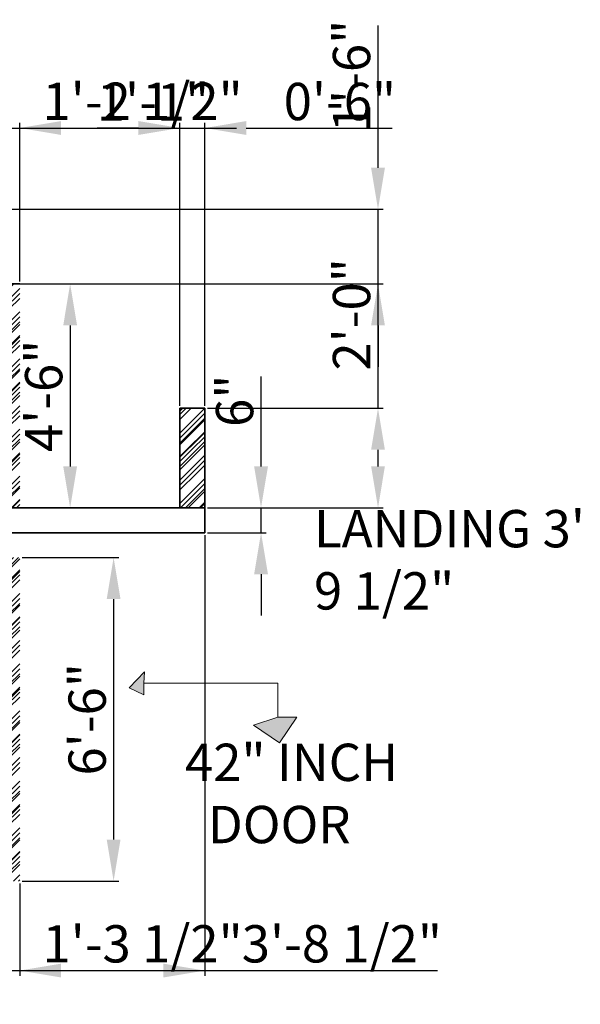
# Model space of a CAD drawing. Units: inches. Extents: x -571 to -216, y 105 to 370.
# Tile 2 of 2: x -351 to -216, y 132 to 370. Entities that reach past the tile are written whole.
import ezdxf

# ---------------------------------------------------------------- set-up
doc = ezdxf.new("R2010")
doc.units = ezdxf.units.IN
for name, color, linetype, lineweight in [('A-ANNO-DIMS', 2, 'Continuous', 18), ('A-ANNO-SYMB', 3, 'Continuous', 18), ('A-ANNO-TEXT', 7, 'Continuous', 18), ('A-FLOR-STRS', 7, 'Continuous', 35), ('A-WALL-PATT', 8, 'Continuous', 18)]:
    doc.layers.add(name, color=color, linetype=linetype, lineweight=lineweight)
doc.styles.get("Standard").update_dxf_attribs({"font": 'arial.ttf'})
doc.dimstyles.new('ISO-25', dxfattribs={"dimtxt": 9, "dimasz": 10, "dimexe": 1.25, "dimexo": 0.625, "dimtad": 1, "dimdec": 0, "dimlunit": 3, "dimtxsty": 'Standard', "dimcen": 2.5, "dimadec": 0, "dimazin": 0, "dimtfac": 1, "dimtdec": 0, "dimtmove": 0, "dimatfit": 3, "dimfxl": 1, "dimarcsym": 0})

# ---------------------------------------------------------------- blocks, each defined once
blk = doc.blocks.new('*D1')
at = {"layer": 'A-ANNO-DIMS', "color": 0, "lineweight": -2, "transparency": 16777216}
for p, q in [((-350.83, 305.84), (-338.04, 305.84)), ((-339.29, 295.84), (-339.29, 261.84)), ((-350.83, 251.84), (-338.04, 251.84))]:
    blk.add_line(p, q, dxfattribs=at)
at = {"layer": 'A-ANNO-DIMS', "color": 0, "transparency": 16777216}
for points in [[(-340.95, 295.84), (-337.62, 295.84), (-339.29, 305.84)], [(-340.95, 261.84), (-337.62, 261.84), (-339.29, 251.84)]]:
    blk.add_solid(points, dxfattribs=at)
at = {"layer": 'Defpoints', "color": 0, "transparency": 16777216}
for p in [(-351.46, 305.84), (-351.46, 251.84), (-339.29, 251.84)]:
    blk.add_point(p, dxfattribs=at)
at = {"layer": 'A-ANNO-DIMS', "color": 0, "transparency": 16777216, "insert": (-344.51, 278.84), "char_height": 9, "attachment_point": 5, "rotation": 90}
blk.add_mtext('4\'-6"', dxfattribs=at)
blk = doc.blocks.new('*D3')
at = {"layer": 'A-ANNO-DIMS', "color": 0, "lineweight": -2, "transparency": 16777216}
for p, q in [((-350.83, 239.84), (-327.55, 239.84)), ((-328.8, 229.84), (-328.8, 171.84)), ((-350.83, 161.84), (-327.55, 161.84))]:
    blk.add_line(p, q, dxfattribs=at)
at = {"layer": 'A-ANNO-DIMS', "color": 0, "transparency": 16777216}
for points in [[(-330.47, 229.84), (-327.13, 229.84), (-328.8, 239.84)], [(-330.47, 171.84), (-327.13, 171.84), (-328.8, 161.84)]]:
    blk.add_solid(points, dxfattribs=at)
at = {"layer": 'Defpoints', "color": 0, "transparency": 16777216}
for p in [(-351.46, 239.84), (-351.46, 161.84), (-328.8, 161.84)]:
    blk.add_point(p, dxfattribs=at)
at = {"layer": 'A-ANNO-DIMS', "color": 0, "transparency": 16777216, "insert": (-334.02, 200.84), "char_height": 9, "attachment_point": 5, "rotation": 90}
blk.add_mtext('6\'-6"', dxfattribs=at)
blk = doc.blocks.new('*D4')
at = {"layer": 'A-ANNO-DIMS', "color": 0, "lineweight": -2, "transparency": 16777216}
for p, q in [((-293.23, 261.84), (-293.23, 283.48)), ((-306.17, 251.84), (-291.98, 251.84)), ((-293.23, 245.84), (-293.23, 251.84)), ((-306.17, 245.84), (-291.98, 245.84)), ((-293.23, 235.84), (-293.23, 225.84))]:
    blk.add_line(p, q, dxfattribs=at)
at = {"layer": 'A-ANNO-DIMS', "color": 0, "transparency": 16777216}
for points in [[(-294.9, 261.84), (-291.56, 261.84), (-293.23, 251.84)], [(-294.9, 235.84), (-291.56, 235.84), (-293.23, 245.84)]]:
    blk.add_solid(points, dxfattribs=at)
at = {"layer": 'Defpoints', "color": 0, "transparency": 16777216}
for p in [(-306.8, 251.84), (-293.23, 251.84), (-306.8, 245.84)]:
    blk.add_point(p, dxfattribs=at)
at = {"layer": 'A-ANNO-DIMS', "color": 0, "transparency": 16777216, "insert": (-298.45, 277.66), "char_height": 9, "attachment_point": 5, "rotation": 90}
blk.add_mtext('6"', dxfattribs=at)
blk = doc.blocks.new('*D18')
at = {"layer": 'A-ANNO-DIMS', "color": 0, "lineweight": -2, "transparency": 16777216}
for p, q in [((-378.71, 259.52), (-378.71, 344.69)), ((-364.46, 306.46), (-364.46, 344.69)), ((-388.71, 343.44), (-398.71, 343.44)), ((-378.71, 343.44), (-364.46, 343.44)), ((-354.46, 343.44), (-299.16, 343.44))]:
    blk.add_line(p, q, dxfattribs=at)
at = {"layer": 'A-ANNO-DIMS', "color": 0, "transparency": 16777216}
for points in [[(-388.71, 345.11), (-388.71, 341.77), (-378.71, 343.44)], [(-354.46, 345.11), (-354.46, 341.77), (-364.46, 343.44)]]:
    blk.add_solid(points, dxfattribs=at)
at = {"layer": 'Defpoints', "color": 0, "transparency": 16777216}
for p in [(-364.46, 343.44), (-364.46, 305.84), (-378.71, 258.89)]:
    blk.add_point(p, dxfattribs=at)
at = {"layer": 'A-ANNO-DIMS', "color": 0, "transparency": 16777216, "insert": (-321.81, 348.72), "char_height": 9, "attachment_point": 5}
blk.add_mtext('1\'-2 1/2"', dxfattribs=at)
blk = doc.blocks.new('*D19')
at = {"layer": 'A-ANNO-DIMS', "color": 0, "lineweight": -2, "transparency": 16777216}
for p, q in [((-364.46, 306.46), (-364.46, 344.69)), ((-351.46, 306.46), (-351.46, 344.69)), ((-374.46, 343.44), (-384.46, 343.44)), ((-364.46, 343.44), (-351.46, 343.44)), ((-341.46, 343.44), (-307.13, 343.44))]:
    blk.add_line(p, q, dxfattribs=at)
at = {"layer": 'A-ANNO-DIMS', "color": 0, "transparency": 16777216}
for points in [[(-374.46, 345.11), (-374.46, 341.77), (-364.46, 343.44)], [(-341.46, 345.11), (-341.46, 341.77), (-351.46, 343.44)]]:
    blk.add_solid(points, dxfattribs=at)
at = {"layer": 'Defpoints', "color": 0, "transparency": 16777216}
for p in [(-351.46, 343.44), (-364.46, 305.84), (-351.46, 305.84)]:
    blk.add_point(p, dxfattribs=at)
at = {"layer": 'A-ANNO-DIMS', "color": 0, "transparency": 16777216, "insert": (-319.3, 348.58), "char_height": 9, "attachment_point": 5}
blk.add_mtext('1\'-1"', dxfattribs=at)
blk = doc.blocks.new('*D20')
at = {"layer": 'A-ANNO-DIMS', "color": 0, "lineweight": -2, "transparency": 16777216}
for p, q in [((-306.8, 245.21), (-306.8, 138.99)), ((-351.46, 161.21), (-351.46, 138.99)), ((-341.46, 140.24), (-316.8, 140.24)), ((-306.8, 140.24), (-250.66, 140.24))]:
    blk.add_line(p, q, dxfattribs=at)
at = {"layer": 'A-ANNO-DIMS', "color": 0, "transparency": 16777216}
for points in [[(-341.46, 141.91), (-341.46, 138.57), (-351.46, 140.24)], [(-316.8, 141.91), (-316.8, 138.57), (-306.8, 140.24)]]:
    blk.add_solid(points, dxfattribs=at)
at = {"layer": 'Defpoints', "color": 0, "transparency": 16777216}
for p in [(-306.8, 245.84), (-351.46, 161.84), (-306.8, 140.24)]:
    blk.add_point(p, dxfattribs=at)
at = {"layer": 'A-ANNO-DIMS', "color": 0, "transparency": 16777216, "insert": (-273.73, 145.52), "char_height": 9, "attachment_point": 5}
blk.add_mtext('3\'-8 1/2"', dxfattribs=at)
blk = doc.blocks.new('*D21')
at = {"layer": 'A-ANNO-DIMS', "color": 0, "lineweight": -2, "transparency": 16777216}
for p, q in [((-265.01, 333.84), (-265.01, 368.17)), ((-451.83, 323.84), (-263.76, 323.84)), ((-265.01, 305.84), (-265.01, 323.84)), ((-451.83, 305.84), (-263.76, 305.84)), ((-265.01, 295.84), (-265.01, 285.84))]:
    blk.add_line(p, q, dxfattribs=at)
at = {"layer": 'A-ANNO-DIMS', "color": 0, "transparency": 16777216}
for points in [[(-266.68, 333.84), (-263.35, 333.84), (-265.01, 323.84)], [(-266.68, 295.84), (-263.35, 295.84), (-265.01, 305.84)]]:
    blk.add_solid(points, dxfattribs=at)
at = {"layer": 'Defpoints', "color": 0, "transparency": 16777216}
for p in [(-452.46, 323.84), (-265.01, 323.84), (-452.46, 305.84)]:
    blk.add_point(p, dxfattribs=at)
at = {"layer": 'A-ANNO-DIMS', "color": 0, "transparency": 16777216, "insert": (-270.23, 356), "char_height": 9, "attachment_point": 5, "rotation": 90}
blk.add_mtext('1\'-6"', dxfattribs=at)
blk = doc.blocks.new('*D24')
at = {"layer": 'A-ANNO-DIMS', "color": 0, "lineweight": -2, "transparency": 16777216}
for p, q in [((-312.8, 276.46), (-312.8, 344.69)), ((-306.8, 276.46), (-306.8, 344.69)), ((-322.8, 343.44), (-332.8, 343.44)), ((-312.8, 343.44), (-306.8, 343.44)), ((-296.8, 343.44), (-261.62, 343.44))]:
    blk.add_line(p, q, dxfattribs=at)
at = {"layer": 'A-ANNO-DIMS', "color": 0, "transparency": 16777216}
for points in [[(-322.8, 345.11), (-322.8, 341.77), (-312.8, 343.44)], [(-296.8, 345.11), (-296.8, 341.77), (-306.8, 343.44)]]:
    blk.add_solid(points, dxfattribs=at)
at = {"layer": 'Defpoints', "color": 0, "transparency": 16777216}
for p in [(-306.8, 343.44), (-312.8, 275.84), (-306.8, 275.84)]:
    blk.add_point(p, dxfattribs=at)
at = {"layer": 'A-ANNO-DIMS', "color": 0, "transparency": 16777216, "insert": (-274.21, 348.66), "char_height": 9, "attachment_point": 5}
blk.add_mtext('0\'-6"', dxfattribs=at)
blk = doc.blocks.new('*D25')
at = {"layer": 'A-ANNO-DIMS', "color": 0, "lineweight": -2, "transparency": 16777216}
for p, q in [((-265.01, 275.84), (-265.01, 311.17)), ((-306.17, 275.84), (-263.76, 275.84)), ((-265.01, 261.84), (-265.01, 265.84)), ((-306.17, 251.84), (-263.76, 251.84))]:
    blk.add_line(p, q, dxfattribs=at)
at = {"layer": 'A-ANNO-DIMS', "color": 0, "transparency": 16777216}
for points in [[(-266.68, 265.84), (-263.35, 265.84), (-265.01, 275.84)], [(-266.68, 261.84), (-263.35, 261.84), (-265.01, 251.84)]]:
    blk.add_solid(points, dxfattribs=at)
at = {"layer": 'Defpoints', "color": 0, "transparency": 16777216}
for p in [(-306.8, 275.84), (-265.01, 275.84), (-306.8, 251.84)]:
    blk.add_point(p, dxfattribs=at)
at = {"layer": 'A-ANNO-DIMS', "color": 0, "transparency": 16777216, "insert": (-270.23, 298.5), "char_height": 9, "attachment_point": 5, "rotation": 90}
blk.add_mtext('2\'-0"', dxfattribs=at)
blk = doc.blocks.new('*D26')
at = {"layer": 'A-ANNO-DIMS', "color": 0, "lineweight": -2, "transparency": 16777216}
for p, q in [((-380.19, 245.21), (-380.19, 138.99)), ((-364.46, 245.21), (-364.46, 138.99)), ((-390.19, 140.24), (-400.19, 140.24)), ((-380.19, 140.24), (-364.46, 140.24)), ((-354.46, 140.24), (-299.16, 140.24))]:
    blk.add_line(p, q, dxfattribs=at)
at = {"layer": 'A-ANNO-DIMS', "color": 0, "transparency": 16777216}
for points in [[(-390.19, 141.91), (-390.19, 138.57), (-380.19, 140.24)], [(-354.46, 141.91), (-354.46, 138.57), (-364.46, 140.24)]]:
    blk.add_solid(points, dxfattribs=at)
at = {"layer": 'Defpoints', "color": 0, "transparency": 16777216}
for p in [(-380.19, 245.84), (-364.46, 245.84), (-364.46, 140.24)]:
    blk.add_point(p, dxfattribs=at)
at = {"layer": 'A-ANNO-DIMS', "color": 0, "transparency": 16777216, "insert": (-321.81, 145.52), "char_height": 9, "attachment_point": 5}
blk.add_mtext('1\'-3 1/2"', dxfattribs=at)

msp = doc.modelspace()

# ---------------------------------------------------------------- hatches: boundary and pattern name
at = {"layer": 'A-ANNO-SYMB'}
h = msp.add_hatch(color=256, dxfattribs=at)
h.dxf.hatch_style = 1
h.paths.add_polyline_path([(-321.53, 209.53), (-321.36, 212.31), (-325.07, 208.42), (-321.53, 206.76)])
h = msp.add_hatch(color=256, dxfattribs=at)
h.dxf.hatch_style = 1
h.paths.add_polyline_path([(-288.8, 195.17), (-284.61, 201.33), (-289.19, 201.33), (-295.07, 199.43)])
at = {"layer": 'A-WALL-PATT'}
h = msp.add_hatch(dxfattribs=at)
h.set_pattern_fill('GOST_GROUND', color=256)
h.paths.add_polyline_path([(-351.46, 305.84), (-364.46, 305.84), (-364.46, 251.84), (-351.46, 251.84)])
h.paths.add_polyline_path([(-351.46, 239.84), (-364.46, 239.84), (-364.46, 161.84), (-351.46, 161.84)])
h.paths.add_polyline_path([(-306.8, 275.84), (-312.8, 275.84), (-312.8, 251.84), (-306.8, 251.84)])
h.paths.add_polyline_path([(-452.46, 323.84), (-465.46, 323.84), (-465.46, 305.84), (-452.46, 305.84)])
h = msp.add_hatch(dxfattribs=at)
h.set_pattern_fill('GOST_GROUND', color=256, scale=0.4)
h.paths.add_polyline_path([(-351.46, 305.84), (-364.46, 305.84), (-364.46, 251.84), (-351.46, 251.84)])
h.paths.add_polyline_path([(-351.46, 239.84), (-364.46, 239.84), (-364.46, 161.84), (-351.46, 161.84)])
h.paths.add_polyline_path([(-452.46, 323.84), (-465.46, 323.84), (-465.46, 305.84), (-452.46, 305.84)])
h.paths.add_polyline_path([(-306.8, 275.84), (-312.8, 275.84), (-312.8, 251.84), (-306.8, 251.84)])

# ---------------------------------------------------------------- linework, layer by layer
at = {"layer": 'A-ANNO-SYMB'}
for p, q in [((-325.07, 208.42), (-321.36, 212.31)), ((-321.36, 212.31), (-321.53, 209.53)), ((-321.53, 209.53), (-289.19, 209.53)), ((-321.53, 209.53), (-321.53, 206.76)), ((-289.19, 209.53), (-289.19, 201.33)), ((-321.53, 206.76), (-325.07, 208.42)), ((-295.07, 199.43), (-289.19, 201.33)), ((-289.19, 201.33), (-284.61, 201.33)), ((-284.61, 201.33), (-288.8, 195.17)), ((-288.8, 195.17), (-295.07, 199.43))]:
    msp.add_line(p, q, dxfattribs=at)
at = {"layer": 'A-FLOR-STRS'}
for points in [[(-364.46, 305.84), (-351.46, 305.84), (-364.46, 305.84), (-364.46, 251.84), (-306.8, 251.84), (-306.8, 275.84), (-312.8, 275.84), (-312.8, 251.84)], [(-490.22, 161.84), (-380.19, 245.84), (-306.8, 245.84), (-306.8, 251.84)]]:
    msp.add_lwpolyline(points, dxfattribs=at)

# ---------------------------------------------------------------- texts
at = {"layer": 'A-ANNO-TEXT', "char_height": 9, "attachment_point": 1}
for s, insert, width in [('\\A1;{\\fArial|b1|i0|c0|p34;LANDING 3\'\\P9 1/2"  }', (-280.45, 251.31), 89.8159), ('{\\fArial|b1|i0|c0|p34;42" INCH \\P  DOOR}', (-311.58, 194.96), 137.2162)]:
    msp.add_mtext(s, dxfattribs=dict(at, insert=insert, width=width))

# ---------------------------------------------------------------- dimensions: what is measured, and where the dimension line sits
at = {"layer": 'A-ANNO-DIMS'}
for base, p1, p2, override, picture, middle in [((-265.01, 323.84), (-452.46, 305.84), (-452.46, 323.84), {"dimdec": 1, "dimlfac": 1, "dimrnd": 0, "dimzin": 1, "dimdsep": 46, "dimlunit": 4, "dimfrac": 2}, '*D21', (-270.23, 356)), ((-265.01, 275.84), (-306.8, 251.84), (-306.8, 275.84), {"dimdec": 1, "dimlfac": 1, "dimrnd": 0, "dimzin": 1, "dimdsep": 46, "dimlunit": 4, "dimfrac": 2}, '*D25', (-270.23, 298.5)), ((-339.29, 251.84), (-351.46, 305.84), (-351.46, 251.84), {"dimclrd": 0, "dimclre": 0, "dimclrt": 0}, '*D1', (-344.51, 278.84)), ((-293.23, 251.84), (-306.8, 245.84), (-306.8, 251.84), {"dimclrd": 0, "dimclre": 0, "dimclrt": 0}, '*D4', (-298.45, 277.66)), ((-328.8, 161.84), (-351.46, 239.84), (-351.46, 161.84), {"dimclrd": 0, "dimclre": 0, "dimclrt": 0}, '*D3', (-334.02, 200.84))]:
    dim = msp.add_linear_dim(base=base, p1=p1, p2=p2, angle=90, dimstyle='ISO-25', override=override, dxfattribs=at)
    dim.commit()
    dim.dimension.update_dxf_attribs({"geometry": picture, "text_midpoint": middle})
for base, p1, p2, picture, middle in [((-364.4597, 343.4398), (-378.7134, 258.8936), (-364.4597, 305.8398), '*D18', (-321.8105, 348.7183)), ((-351.46, 343.44), (-364.46, 305.84), (-351.46, 305.84), '*D19', (-319.3, 348.58)), ((-306.8, 343.44), (-312.8, 275.84), (-306.8, 275.84), '*D24', (-274.21, 348.66)), ((-364.46, 140.24), (-380.19, 245.84), (-364.46, 245.84), '*D26', (-321.81, 145.52)), ((-306.8, 140.24), (-351.46, 161.84), (-306.8, 245.84), '*D20', (-273.73, 145.52))]:
    dim = msp.add_linear_dim(base=base, p1=p1, p2=p2, dimstyle='ISO-25', override={"dimdec": 1, "dimlfac": 1, "dimrnd": 0, "dimzin": 1, "dimdsep": 46, "dimlunit": 4, "dimfrac": 2}, dxfattribs=at)
    dim.commit()
    dim.dimension.update_dxf_attribs({"geometry": picture, "text_midpoint": middle})

doc.saveas('drawing.dxf')
